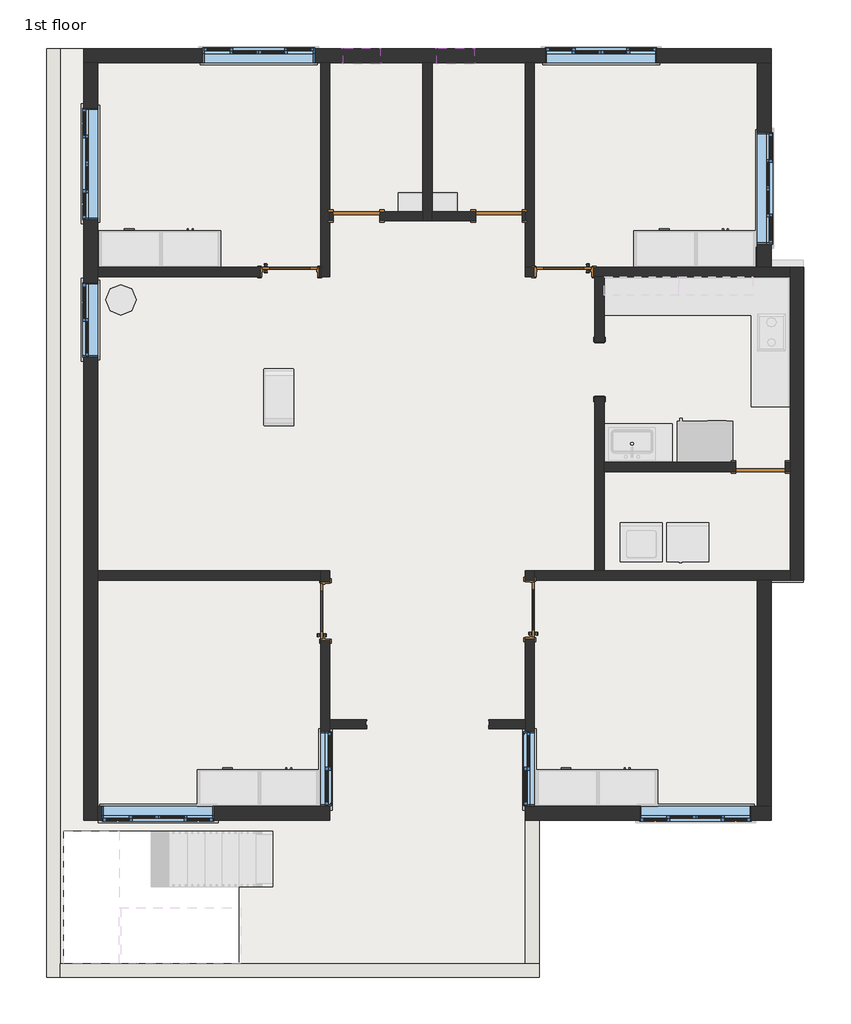
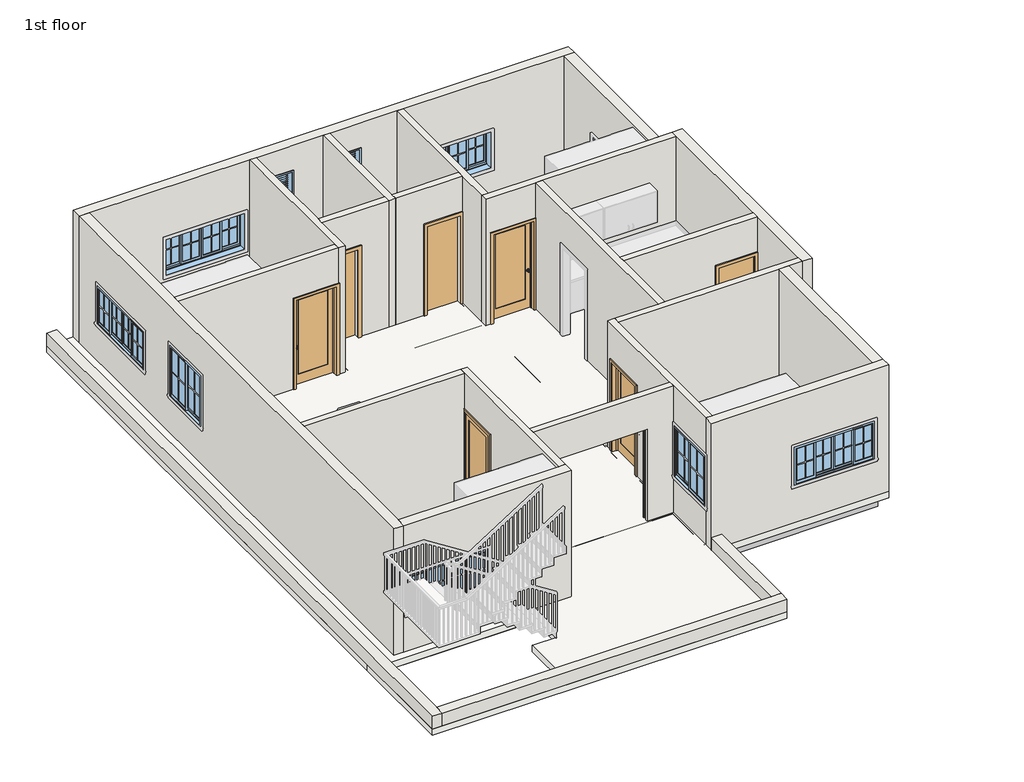
# One storey, part 1 of 4: 24 walls, 11 windows, 7 beams, 7 doors, 1 slab.
"""IFC4 building model written with IfcOpenShell, lengths in millimetres."""

from ifc_helpers import new_model, si_unit, frame, origin, place, context, project, spatial, polyline, outline, extrude, faceted_brep, transform, mapped, element, save
from components import door_010cc4d9, door_5a860750, door_e2b13fe9, door_a9addea7, door_bb092f7c, window_f2d8fef0, window_c1e3dfc0, window_49fe3060, window_58cce754

model = new_model("IFC4")

# Units and contexts
model_context = context("Model", 3, world=origin())
ifc_project = project(units=[si_unit("LENGTHUNIT", "METRE", prefix="MILLI")], contexts=[model_context])

# Site, building, storey
site = spatial("IfcSite", under=ifc_project)
building = spatial("IfcBuilding", under=site)
storey = spatial("IfcBuildingStorey", under=building, Name="1st floor", Elevation=3810.0)

# Beams
placement = place(None, origin())
element("IfcBeam", 1, ObjectType="Concrete-Rectangular Beam", at=placement, inside=storey, context=model_context, shape_type="SweptSolid", body=[
    extrude(outline(polyline([(-1593.2124084, 1316.1961804), (-1364.6124084, 1316.1961804), (-1364.6124084, -2163.6038196), (-1593.2124084, -2163.6038196), (-1593.2124084, 1316.1961804)])), frame((0.0, 0.0, 3505.2), z_axis=(0.0, 0.0, 1.0), x_axis=(1.0, 0.0, 0.0)), (0.0, 0.0, 1.0), 304.8),
])
element("IfcBeam", 2, ObjectType="Concrete-Rectangular Beam", at=placement, inside=storey, context=model_context, shape_type="Brep", body=[
    faceted_brep([(-1593.2124084, -2201.7038196, 3810.0), (-5212.7124084, -2201.7038196, 3810.0), (-5441.3124084, -2201.7038196, 3810.0), (-5441.3124084, -2239.8038196, 3810.0), (-5174.6124084, -2239.8038196, 3810.0), (-5174.6124084, -2430.3038196, 3810.0), (-1593.2124084, -2430.3038196, 3810.0), (-1593.2124084, -2201.7038196, 3505.2), (-5212.7124084, -2201.7038196, 3505.2), (-5441.3124084, -2201.7038196, 3505.2), (-1593.2124084, -2430.3038196, 3505.2), (-5174.6124084, -2430.3038196, 3505.2), (-5174.6124084, -2239.8038196, 3505.2), (-5441.3124084, -2239.8038196, 3505.2)], [[[0, 1, 2, 3, 4, 5, 6]], [[0, 7, 8, 9, 2, 1]], [[9, 8, 7, 10, 11, 12, 13]], [[10, 6, 5, 11]], [[7, 0, 6, 10]], [[2, 9, 13, 3]], [[12, 4, 3, 13]], [[4, 12, 11, 5]]]),
])
element("IfcBeam", 3, ObjectType="Concrete-Rectangular Beam", at=placement, inside=storey, context=model_context, shape_type="Brep", body=[
    faceted_brep([(-8756.0124084, -2468.4038196, 3810.0), (-8756.0124084, -2239.8038196, 3810.0), (-8794.1124084, -2239.8038196, 3810.0), (-12413.6124084, -2239.8038196, 3810.0), (-12413.6124084, -2468.4038196, 3810.0), (-8756.0124084, -2239.8038196, 3505.2), (-8794.1124084, -2239.8038196, 3505.2), (-12413.6124084, -2239.8038196, 3505.2), (-8756.0124084, -2468.4038196, 3505.2), (-12413.6124084, -2468.4038196, 3505.2)], [[[0, 1, 2, 3, 4]], [[1, 5, 6, 7, 3, 2]], [[5, 8, 9, 7, 6]], [[8, 0, 4, 9]], [[1, 0, 8, 5]], [[4, 3, 7, 9]]]),
])
element("IfcBeam", 4, ObjectType="Concrete-Rectangular Beam", at=placement, inside=storey, context=model_context, shape_type="SweptSolid", body=[
    extrude(outline(polyline([(-12642.2124084, 9875.9961804), (-12413.6124084, 9875.9961804), (-12413.6124084, 6751.7961804), (-12642.2124084, 6751.7961804), (-12642.2124084, 9875.9961804)])), frame((0.0, 0.0, 3505.2), z_axis=(0.0, 0.0, 1.0), x_axis=(1.0, 0.0, 0.0)), (0.0, 0.0, 1.0), 304.8),
    extrude(outline(polyline([(-12413.6124084, -2163.6038196), (-12642.2124084, -2163.6038196), (-12642.2124084, 1392.3961804), (-12413.6124084, 1392.3961804), (-12413.6124084, -2163.6038196)])), frame((0.0, 0.0, 3505.2), z_axis=(0.0, 0.0, 1.0), x_axis=(1.0, 0.0, 0.0)), (0.0, 0.0, 1.0), 304.8),
    extrude(outline(polyline([(-12413.6124084, 1697.1961804), (-12642.2124084, 1697.1961804), (-12642.2124084, 6446.9961804), (-12413.6124084, 6446.9961804), (-12413.6124084, 1697.1961804)])), frame((0.0, 0.0, 3505.2), z_axis=(0.0, 0.0, 1.0), x_axis=(1.0, 0.0, 0.0)), (0.0, 0.0, 1.0), 304.8),
])
element("IfcBeam", 5, ObjectType="Concrete-Rectangular Beam", at=placement, inside=storey, context=model_context, shape_type="Brep", body=[
    faceted_brep([(-843.9124084, 1659.0961804, 3810.0), (-843.9124084, 1430.4961804, 3810.0), (-843.9124084, 1430.4961804, 3505.2), (-843.9124084, 1659.0961804, 3505.2), (-5098.4124084, 1659.0961804, 3810.0), (-5098.4124084, 1468.5961804, 3810.0), (-5403.2124084, 1468.5961804, 3810.0), (-5403.2124084, 1659.0961804, 3810.0), (-5441.3124084, 1659.0961804, 3810.0), (-8565.5124084, 1659.0961804, 3810.0), (-8603.6124084, 1659.0961804, 3810.0), (-8603.6124084, 1468.5961804, 3810.0), (-8908.4124084, 1468.5961804, 3810.0), (-8908.4124084, 1659.0961804, 3810.0), (-12413.6124084, 1659.0961804, 3810.0), (-12413.6124084, 1430.4961804, 3810.0), (-8794.1124084, 1430.4961804, 3810.0), (-8565.5124084, 1430.4961804, 3810.0), (-5441.3124084, 1430.4961804, 3810.0), (-5212.7124084, 1430.4961804, 3810.0), (-1593.2124084, 1430.4961804, 3810.0), (-1593.2124084, 1620.9961804, 3810.0), (-1364.6124084, 1620.9961804, 3810.0), (-1364.6124084, 1430.4961804, 3810.0), (-1364.6124084, 1430.4961804, 3505.2), (-1364.6124084, 1620.9961804, 3505.2), (-1593.2124084, 1620.9961804, 3505.2), (-1593.2124084, 1430.4961804, 3505.2), (-5212.7124084, 1430.4961804, 3505.2), (-5441.3124084, 1430.4961804, 3505.2), (-8565.5124084, 1430.4961804, 3505.2), (-8794.1124084, 1430.4961804, 3505.2), (-12413.6124084, 1430.4961804, 3505.2), (-12413.6124084, 1659.0961804, 3505.2), (-8908.4124084, 1659.0961804, 3505.2), (-8908.4124084, 1468.5961804, 3505.2), (-8603.6124084, 1468.5961804, 3505.2), (-8603.6124084, 1659.0961804, 3505.2), (-8565.5124084, 1659.0961804, 3505.2), (-5441.3124084, 1659.0961804, 3505.2), (-5403.2124084, 1659.0961804, 3505.2), (-5403.2124084, 1468.5961804, 3505.2), (-5098.4124084, 1468.5961804, 3505.2), (-5098.4124084, 1659.0961804, 3505.2)], [[[0, 1, 2, 3]], [[1, 0, 4, 5, 6, 7, 8, 9, 10, 11, 12, 13, 14, 15, 16, 17, 18, 19, 20, 21, 22, 23]], [[2, 1, 23, 24]], [[3, 2, 24, 25, 26, 27, 28, 29, 30, 31, 32, 33, 34, 35, 36, 37, 38, 39, 40, 41, 42, 43]], [[0, 3, 43, 4]], [[15, 14, 33, 32]], [[22, 25, 24, 23]], [[26, 21, 20, 27]], [[21, 26, 25, 22]], [[15, 32, 31, 30, 29, 28, 27, 20, 19, 18, 17, 16]], [[36, 11, 10, 37]], [[11, 36, 35, 12]], [[12, 35, 34, 13]], [[33, 14, 13, 34]], [[42, 5, 4, 43]], [[5, 42, 41, 6]], [[6, 41, 40, 7]], [[37, 10, 9, 8, 7, 40, 39, 38]]]),
])
element("IfcBeam", 6, ObjectType="Concrete-Rectangular Beam", at=placement, inside=storey, context=model_context, shape_type="Brep", body=[
    faceted_brep([(-8794.1124084, -2239.8038196, 3810.0), (-8756.0124084, -2239.8038196, 3810.0), (-8565.5124084, -2239.8038196, 3810.0), (-8565.5124084, -1007.9038196, 3810.0), (-8565.5124084, -779.3038196, 3810.0), (-8565.5124084, 1430.4961804, 3810.0), (-8794.1124084, 1430.4961804, 3810.0), (-8794.1124084, -2239.8038196, 3505.2), (-8794.1124084, 1430.4961804, 3505.2), (-8565.5124084, -2239.8038196, 3505.2), (-8756.0124084, -2239.8038196, 3505.2), (-8565.5124084, 1430.4961804, 3505.2), (-8565.5124084, -779.3038196, 3505.2), (-8565.5124084, -1007.9038196, 3505.2)], [[[0, 1, 2, 3, 4, 5, 6]], [[7, 0, 6, 8]], [[9, 10, 7, 8, 11, 12, 13]], [[11, 5, 4, 3, 2, 9, 13, 12]], [[2, 1, 0, 7, 10, 9]], [[5, 11, 8, 6]]]),
    faceted_brep([(-8794.1124084, 9914.0961804, 3810.0), (-8565.5124084, 9914.0961804, 3810.0), (-8565.5124084, 9914.0961804, 3505.2), (-8794.1124084, 9914.0961804, 3505.2), (-8794.1124084, 6713.6961804, 3810.0), (-8794.1124084, 6713.6961804, 3505.2), (-8756.0124084, 6713.6961804, 3505.2), (-8756.0124084, 6713.6961804, 3810.0), (-8756.0124084, 6751.7961804, 3810.0), (-8565.5124084, 6751.7961804, 3810.0), (-8565.5124084, 7323.2961804, 3810.0), (-8565.5124084, 7551.8961804, 3810.0), (-8565.5124084, 7551.8961804, 3505.2), (-8565.5124084, 7323.2961804, 3505.2), (-8565.5124084, 6751.7961804, 3505.2), (-8756.0124084, 6751.7961804, 3505.2)], [[[0, 1, 2, 3]], [[4, 5, 6, 7]], [[1, 0, 4, 7, 8, 9, 10, 11]], [[3, 2, 12, 13, 14, 15, 6, 5]], [[0, 3, 5, 4]], [[2, 1, 11, 10, 9, 14, 13, 12]], [[15, 8, 7, 6]], [[8, 15, 14, 9]]]),
    faceted_brep([(-8794.1124084, 6485.0961804, 3505.2), (-8794.1124084, 6485.0961804, 3810.0), (-8756.0124084, 6485.0961804, 3810.0), (-8756.0124084, 6485.0961804, 3505.2), (-8565.5124084, 1659.0961804, 3505.2), (-8565.5124084, 1659.0961804, 3810.0), (-8603.6124084, 1659.0961804, 3810.0), (-8603.6124084, 1659.0961804, 3505.2), (-8565.5124084, 6446.9961804, 3505.2), (-8565.5124084, 6446.9961804, 3810.0), (-8794.1124084, 1697.1961804, 3810.0), (-8603.6124084, 1697.1961804, 3810.0), (-8756.0124084, 6446.9961804, 3810.0), (-8794.1124084, 1697.1961804, 3505.2), (-8603.6124084, 1697.1961804, 3505.2), (-8756.0124084, 6446.9961804, 3505.2)], [[[0, 1, 2, 3]], [[4, 5, 6, 7]], [[5, 4, 8, 9]], [[2, 1, 10, 11, 6, 5, 9, 12]], [[1, 0, 13, 10]], [[8, 4, 7, 14, 13, 0, 3, 15]], [[15, 12, 9, 8]], [[12, 15, 3, 2]], [[14, 11, 10, 13]], [[11, 14, 7, 6]]]),
])
element("IfcBeam", 7, ObjectType="Concrete-Rectangular Beam", at=placement, inside=storey, context=model_context, shape_type="SweptSolid", body=[
    extrude(outline(polyline([(-5441.3124084, -779.3038196), (-5441.3124084, -1007.9038196), (-8565.5124084, -1007.9038196), (-8565.5124084, -779.3038196), (-5441.3124084, -779.3038196)])), frame((0.0, 0.0, 3505.2), z_axis=(0.0, 0.0, 1.0), x_axis=(1.0, 0.0, 0.0)), (0.0, 0.0, 1.0), 304.8),
])

# Doors
door_shape = door_010cc4d9(model_context)
element("IfcDoor", 8, ObjectType="Door-Interior-Single-1_Panel-Wood : 36\" x 84\"", at=placement, inside=storey, context=model_context, shape_type="MappedRepresentation", body=[
    mapped(door_shape, transform((-9264.0124084, 6526.3711804, 3810.0), x_axis=(1.0, 0.0, 0.0), y_axis=(0.0, 1.0, 0.0), z_axis=(0.0, 0.0, 1.0))),
])
element("IfcDoor", 9, ObjectType="Door-Interior-Single-1_Panel-Wood : 36\" x 84\"", at=placement, inside=storey, context=model_context, shape_type="MappedRepresentation", body=[
    mapped(door_shape, transform((-8682.9874084, 960.5961804, 3810.0), x_axis=(0.0, 1.0, 0.0), y_axis=(-1.0, 0.0, 0.0), z_axis=(0.0, 0.0, 1.0))),
])
door_2_shape = door_5a860750(model_context)
element("IfcDoor", 10, ObjectType="Door-Interior-Single-1_Panel-Wood : 36\" x 84\"", at=placement, inside=storey, context=model_context, shape_type="MappedRepresentation", body=[
    mapped(door_2_shape, transform((-4768.2124084, 6526.3711804, 3810.0), x_axis=(-1.0, 0.0, 0.0), y_axis=(0.0, -1.0, 0.0), z_axis=(0.0, 0.0, 1.0))),
])
element("IfcDoor", 11, ObjectType="Door-Interior-Single-1_Panel-Wood : 36\" x 84\"", at=placement, inside=storey, context=model_context, shape_type="MappedRepresentation", body=[
    mapped(door_2_shape, transform((-5323.8374084, 985.9961804, 3810.0), x_axis=(0.0, 1.0, 0.0), y_axis=(-1.0, 0.0, 0.0), z_axis=(0.0, 0.0, 1.0))),
])
door_3_shape = door_e2b13fe9(model_context)
element("IfcDoor", 12, ObjectType="Single-Flush : 30\" x 84\"", at=placement, inside=storey, context=model_context, shape_type="MappedRepresentation", body=[
    mapped(door_3_shape, transform((-8171.8124084, 7437.5961804, 3810.0), x_axis=(-1.0, 0.0, 0.0), y_axis=(0.0, -1.0, 0.0), z_axis=(0.0, 0.0, 1.0))),
])
door_4_shape = door_a9addea7(model_context)
element("IfcDoor", 13, ObjectType="Single-Flush : 30\" x 84\"", at=placement, inside=storey, context=model_context, shape_type="MappedRepresentation", body=[
    mapped(door_4_shape, transform((-5835.0124084, 7437.5961804, 3810.0), x_axis=(1.0, 0.0, 0.0), y_axis=(0.0, 1.0, 0.0), z_axis=(0.0, 0.0, 1.0))),
])
door_5_shape = door_bb092f7c(model_context)
element("IfcDoor", 14, ObjectType="Single-Flush : 32\" x 84\"", at=placement, inside=storey, context=model_context, shape_type="MappedRepresentation", body=[
    mapped(door_5_shape, transform((-1542.4124084, 3322.7961804, 3810.0), x_axis=(1.0, 0.0, 0.0), y_axis=(0.0, 1.0, 0.0), z_axis=(0.0, 0.0, 1.0))),
])

# Slab
element("IfcSlab", 15, ObjectType="Generic - 6\"", at=placement, inside=storey, context=model_context, shape_type="SweptSolid", body=[
    extrude(outline(polyline([(-1364.6124084, 10180.7961804), (-1364.6124084, 6599.3961804), (-831.2124084, 6599.3961804), (-831.2124084, 1468.5961804), (-1364.6124084, 1468.5961804), (-1364.6124084, -2468.4038196), (-5174.6124084, -2468.4038196), (-5174.6124084, -5046.5038196), (-13251.8124084, -5046.5038196), (-13251.8124084, -2468.4038196), (-13251.8124084, 10180.7961804), (-1364.6124084, 10180.7961804)]), holes=[polyline([(-9543.8120641, -3536.9669819), (-9543.8120641, -2647.9669819), (-12972.8120641, -2647.9669819), (-12972.8120641, -4817.9038196), (-10102.6120641, -4817.9038196), (-10102.6120641, -3536.9669819), (-9543.8120641, -3536.9669819)])]), frame((0.0, 0.0, 3657.6), z_axis=(0.0, 0.0, 1.0), x_axis=(1.0, 0.0, 0.0)), (0.0, 0.0, 1.0), 152.4),
])

# Walls
element("IfcWall", 16, ObjectType="Generic - 6\"", at=placement, inside=storey, context=model_context, shape_type="Brep", body=[
    faceted_brep([(-8756.0124084, 9952.1961804, 3810.0), (-8756.0124084, 6599.3961804, 3810.0), (-8756.0124084, 6446.9961804, 3810.0), (-8756.0124084, 6446.9961804, 6858.0), (-8756.0124084, 6599.3961804, 6858.0), (-8756.0124084, 9952.1961804, 6858.0), (-8603.6124084, 9952.1961804, 3810.0), (-8603.6124084, 9952.1961804, 6858.0), (-8603.6124084, 7513.7961804, 6858.0), (-8603.6124084, 7361.3961804, 6858.0), (-8603.6124084, 6446.9961804, 6858.0), (-8603.6124084, 6446.9961804, 3810.0), (-8603.6124084, 7361.3961804, 3810.0), (-8603.6124084, 7513.7961804, 3810.0)], [[[0, 1, 2, 3, 4, 5]], [[6, 7, 8, 9, 10, 11, 12, 13]], [[2, 1, 0, 6, 13, 12, 11]], [[0, 5, 7, 6]], [[3, 2, 11, 10]], [[5, 4, 3, 10, 9, 8, 7]]]),
])
element("IfcWall", 17, ObjectType="Generic - 6\"", at=placement, inside=storey, context=model_context, shape_type="SweptSolid", body=[
    extrude(outline(polyline([(3810.0, -8756.0124084), (6858.0, -8756.0124084), (6858.0, -12413.6124084), (3810.0, -12413.6124084), (3810.0, -9746.6124084), (5969.0, -9746.6124084), (5969.0, -8781.4124084), (3810.0, -8781.4124084), (3810.0, -8756.0124084)])), frame((0.0, 6446.9961804, 0.0), z_axis=(0.0, 1.0, 0.0), x_axis=(0.0, 0.0, 1.0)), (0.0, 0.0, 1.0), 152.4),
])
element("IfcWall", 18, ObjectType="Generic - 6\"", at=placement, inside=storey, context=model_context, shape_type="Brep", body=[
    faceted_brep([(-7079.6124084, 9952.1961804, 3810.0), (-7079.6124084, 7513.7961804, 3810.0), (-7079.6124084, 7361.3961804, 3810.0), (-7079.6124084, 7361.3961804, 6858.0), (-7079.6124084, 7513.7961804, 6858.0), (-7079.6124084, 9952.1961804, 6858.0), (-6927.2124084, 9952.1961804, 3810.0), (-6927.2124084, 9952.1961804, 6858.0), (-6927.2124084, 7513.7961804, 6858.0), (-6927.2124084, 7361.3961804, 6858.0), (-6927.2124084, 7361.3961804, 3810.0), (-6927.2124084, 7513.7961804, 3810.0)], [[[0, 1, 2, 3, 4, 5]], [[6, 7, 8, 9, 10, 11]], [[2, 1, 0, 6, 11, 10]], [[0, 5, 7, 6]], [[3, 2, 10, 9]], [[5, 4, 3, 9, 8, 7]]]),
])
element("IfcWall", 19, ObjectType="Generic - 6\"", at=placement, inside=storey, context=model_context, shape_type="SweptSolid", body=[
    extrude(outline(polyline([(3810.0, -7079.6124084), (6858.0, -7079.6124084), (6858.0, -8603.6124084), (3810.0, -8603.6124084), (3810.0, -8552.8124084), (5943.6, -8552.8124084), (5943.6, -7790.8124084), (3810.0, -7790.8124084), (3810.0, -7079.6124084)])), frame((0.0, 7361.3961804, 0.0), z_axis=(0.0, 1.0, 0.0), x_axis=(0.0, 0.0, 1.0)), (0.0, 0.0, 1.0), 152.4),
])
element("IfcWall", 20, ObjectType="Generic - 6\"", at=placement, inside=storey, context=model_context, shape_type="SweptSolid", body=[
    extrude(outline(polyline([(6858.0, -6927.2124084), (3810.0, -6927.2124084), (3810.0, -6216.0124084), (5943.6, -6216.0124084), (5943.6, -5454.0124084), (3810.0, -5454.0124084), (3810.0, -5403.2124084), (6858.0, -5403.2124084), (6858.0, -6927.2124084)])), frame((0.0, 7361.3961804, 0.0), z_axis=(0.0, 1.0, 0.0), x_axis=(0.0, 0.0, 1.0)), (0.0, 0.0, 1.0), 152.4),
])
element("IfcWall", 21, ObjectType="Generic - 6\"", at=placement, inside=storey, context=model_context, shape_type="Brep", body=[
    faceted_brep([(-5250.8124084, 6599.3961804, 3810.0), (-5250.8124084, 9952.1961804, 3810.0), (-5250.8124084, 9952.1961804, 6858.0), (-5250.8124084, 6599.3961804, 6858.0), (-5403.2124084, 6599.3961804, 3810.0), (-5403.2124084, 6599.3961804, 6858.0), (-5403.2124084, 7361.3961804, 6858.0), (-5403.2124084, 7513.7961804, 6858.0), (-5403.2124084, 9952.1961804, 6858.0), (-5403.2124084, 9952.1961804, 3810.0), (-5403.2124084, 7513.7961804, 3810.0), (-5403.2124084, 7361.3961804, 3810.0)], [[[0, 1, 2, 3]], [[4, 5, 6, 7, 8, 9, 10, 11]], [[1, 0, 4, 11, 10, 9]], [[2, 1, 9, 8]], [[0, 3, 5, 4]], [[3, 2, 8, 7, 6, 5]]]),
])
element("IfcWall", 22, ObjectType="Generic - 6\"", at=placement, inside=storey, context=model_context, shape_type="Brep", body=[
    faceted_brep([(-5403.2124084, 6599.3961804, 3810.0), (-5403.2124084, 6599.3961804, 6858.0), (-5250.8124084, 6599.3961804, 6858.0), (-1593.2124084, 6599.3961804, 6858.0), (-1364.6124084, 6599.3961804, 6858.0), (-1059.8124084, 6599.3961804, 6858.0), (-1059.8124084, 6599.3961804, 3810.0), (-1364.6124084, 6599.3961804, 3810.0), (-1593.2124084, 6599.3961804, 3810.0), (-4285.6124084, 6599.3961804, 3810.0), (-4285.6124084, 6599.3961804, 5969.0), (-5250.8124084, 6599.3961804, 5969.0), (-5250.8124084, 6599.3961804, 3810.0), (-1059.8124084, 6446.9961804, 6858.0), (-4107.8124084, 6446.9961804, 6858.0), (-4260.2124084, 6446.9961804, 6858.0), (-5403.2124084, 6446.9961804, 6858.0), (-5403.2124084, 6446.9961804, 3810.0), (-5250.8124084, 6446.9961804, 3810.0), (-5250.8124084, 6446.9961804, 5969.0), (-4285.6124084, 6446.9961804, 5969.0), (-4285.6124084, 6446.9961804, 3810.0), (-4260.2124084, 6446.9961804, 3810.0), (-4107.8124084, 6446.9961804, 3810.0), (-1059.8124084, 6446.9961804, 3810.0)], [[[0, 1, 2, 3, 4, 5, 6, 7, 8, 9, 10, 11, 12]], [[13, 14, 15, 16, 17, 18, 19, 20, 21, 22, 23, 24]], [[17, 0, 12, 18]], [[6, 24, 23, 22, 21, 9, 8, 7]], [[1, 0, 17, 16]], [[6, 5, 13, 24]], [[11, 19, 18, 12]], [[19, 11, 10, 20]], [[20, 10, 9, 21]], [[16, 15, 14, 13, 5, 4, 3, 2, 1]]]),
])
element("IfcWall", 23, ObjectType="Generic - 6\"", at=placement, inside=storey, context=model_context, shape_type="SweptSolid", body=[
    extrude(outline(polyline([(-8756.0124084, 1468.5961804), (-12413.6124084, 1468.5961804), (-12413.6124084, 1620.9961804), (-8756.0124084, 1620.9961804), (-8756.0124084, 1468.5961804)])), frame((0.0, 0.0, 3810.0), z_axis=(0.0, 0.0, 1.0), x_axis=(1.0, 0.0, 0.0)), (0.0, 0.0, 1.0), 3048.0),
])
element("IfcWall", 24, ObjectType="Generic - 6\"", at=placement, inside=storey, context=model_context, shape_type="Brep", body=[
    faceted_brep([(-5403.2124084, -2239.8038196, 3810.0), (-5403.2124084, -2239.8038196, 6858.0), (-5403.2124084, -969.8038196, 6858.0), (-5403.2124084, -817.4038196, 6858.0), (-5403.2124084, 1620.9961804, 6858.0), (-5403.2124084, 1620.9961804, 3810.0), (-5403.2124084, 1468.5961804, 3810.0), (-5403.2124084, 1468.5961804, 5969.0), (-5403.2124084, 503.3961804, 5969.0), (-5403.2124084, 503.3961804, 3810.0), (-5403.2124084, -817.4038196, 3810.0), (-5403.2124084, -969.8038196, 3810.0), (-5403.2124084, -1014.2538196, 4724.4), (-5403.2124084, -1014.2538196, 5943.6), (-5403.2124084, -2233.4538196, 5943.6), (-5403.2124084, -2233.4538196, 4724.4), (-5250.8124084, -2239.8038196, 6858.0), (-5250.8124084, -2239.8038196, 3810.0), (-5250.8124084, 503.3961804, 3810.0), (-5250.8124084, 503.3961804, 5969.0), (-5250.8124084, 1468.5961804, 5969.0), (-5250.8124084, 1468.5961804, 3810.0), (-5250.8124084, 1620.9961804, 3810.0), (-5250.8124084, 1620.9961804, 6858.0), (-5250.8124084, 1468.5961804, 6858.0), (-5250.8124084, -1014.2538196, 5943.6), (-5250.8124084, -1014.2538196, 4724.4), (-5250.8124084, -2233.4538196, 4724.4), (-5250.8124084, -2233.4538196, 5943.6)], [[[0, 1, 2, 3, 4, 5, 6, 7, 8, 9, 10, 11], [12, 13, 14, 15]], [[16, 17, 18, 19, 20, 21, 22, 23, 24], [25, 26, 27, 28]], [[17, 0, 11, 10, 9, 18]], [[5, 22, 21, 6]], [[1, 0, 17, 16]], [[5, 4, 23, 22]], [[20, 7, 6, 21]], [[7, 20, 19, 8]], [[8, 19, 18, 9]], [[25, 13, 12, 26]], [[26, 12, 15, 27]], [[27, 15, 14, 28]], [[13, 25, 28, 14]], [[4, 3, 2, 1, 16, 24, 23]]]),
])
element("IfcWall", 25, ObjectType="Generic - 6\"", at=placement, inside=storey, context=model_context, shape_type="Brep", body=[
    faceted_brep([(-8756.0124084, 1620.9961804, 3810.0), (-8756.0124084, 1468.5961804, 3810.0), (-8756.0124084, 1443.1961804, 3810.0), (-8756.0124084, 1443.1961804, 5969.0), (-8756.0124084, 477.9961804, 5969.0), (-8756.0124084, 477.9961804, 3810.0), (-8756.0124084, -2239.8038196, 3810.0), (-8756.0124084, -2239.8038196, 6858.0), (-8756.0124084, 1468.5961804, 6858.0), (-8756.0124084, 1620.9961804, 6858.0), (-8756.0124084, -2233.4538196, 5943.6), (-8756.0124084, -2233.4538196, 4724.4), (-8756.0124084, -1014.2538196, 4724.4), (-8756.0124084, -1014.2538196, 5943.6), (-8603.6124084, 1443.1961804, 3810.0), (-8603.6124084, 1620.9961804, 3810.0), (-8603.6124084, 1620.9961804, 6858.0), (-8603.6124084, -817.4038196, 6858.0), (-8603.6124084, -969.8038196, 6858.0), (-8603.6124084, -2239.8038196, 6858.0), (-8603.6124084, -2239.8038196, 3810.0), (-8603.6124084, -969.8038196, 3810.0), (-8603.6124084, -817.4038196, 3810.0), (-8603.6124084, 477.9961804, 3810.0), (-8603.6124084, 477.9961804, 5969.0), (-8603.6124084, 1443.1961804, 5969.0), (-8603.6124084, -2233.4538196, 4724.4), (-8603.6124084, -2233.4538196, 5943.6), (-8603.6124084, -1014.2538196, 5943.6), (-8603.6124084, -1014.2538196, 4724.4)], [[[0, 1, 2, 3, 4, 5, 6, 7, 8, 9], [10, 11, 12, 13]], [[14, 15, 16, 17, 18, 19, 20, 21, 22, 23, 24, 25], [26, 27, 28, 29]], [[6, 5, 23, 22, 21, 20]], [[2, 1, 0, 15, 14]], [[25, 3, 2, 14]], [[3, 25, 24, 4]], [[4, 24, 23, 5]], [[0, 9, 16, 15]], [[10, 27, 26, 11]], [[11, 26, 29, 12]], [[12, 29, 28, 13]], [[27, 10, 13, 28]], [[9, 8, 7, 19, 18, 17, 16]], [[7, 6, 20, 19]]]),
])
element("IfcWall", 26, ObjectType="Generic - 6\"", at=placement, inside=storey, context=model_context, shape_type="Brep", body=[
    faceted_brep([(-4260.2124084, 6446.9961804, 6858.0), (-4260.2124084, 6446.9961804, 3810.0), (-4260.2124084, 5380.1961804, 3810.0), (-4260.2124084, 5380.1961804, 5943.6), (-4260.2124084, 4465.7961804, 5943.6), (-4260.2124084, 4465.7961804, 3810.0), (-4260.2124084, 1620.9961804, 3810.0), (-4260.2124084, 1620.9961804, 6858.0), (-4107.8124084, 6446.9961804, 3810.0), (-4107.8124084, 6446.9961804, 6858.0), (-4107.8124084, 3398.9961804, 6858.0), (-4107.8124084, 3246.5961804, 6858.0), (-4107.8124084, 1620.9961804, 6858.0), (-4107.8124084, 1620.9961804, 3810.0), (-4107.8124084, 3246.5961804, 3810.0), (-4107.8124084, 3398.9961804, 3810.0), (-4107.8124084, 4465.7961804, 3810.0), (-4107.8124084, 4465.7961804, 5943.6), (-4107.8124084, 5380.1961804, 5943.6), (-4107.8124084, 5380.1961804, 3810.0)], [[[0, 1, 2, 3, 4, 5, 6, 7]], [[8, 9, 10, 11, 12, 13, 14, 15, 16, 17, 18, 19]], [[1, 8, 19, 2]], [[13, 6, 5, 16, 15, 14]], [[1, 0, 9, 8]], [[7, 6, 13, 12]], [[4, 17, 16, 5]], [[18, 3, 2, 19]], [[17, 4, 3, 18]], [[0, 7, 12, 11, 10, 9]]]),
])
element("IfcWall", 27, ObjectType="Generic - 6\"", at=placement, inside=storey, context=model_context, shape_type="SweptSolid", body=[
    extrude(outline(polyline([(6858.0, -4107.8124084), (3810.0, -4107.8124084), (3810.0, -1948.8124084), (5943.6, -1948.8124084), (5943.6, -1136.0124084), (3810.0, -1136.0124084), (3810.0, -1059.8124084), (6858.0, -1059.8124084), (6858.0, -4107.8124084)])), frame((0.0, 3246.5961804, 0.0), z_axis=(0.0, 1.0, 0.0), x_axis=(0.0, 0.0, 1.0)), (0.0, 0.0, 1.0), 152.4),
])
element("IfcWall", 28, ObjectType="Generic - 6\"", at=placement, inside=storey, context=model_context, shape_type="Brep", body=[
    faceted_brep([(-5250.8124084, 1468.5961804, 3810.0), (-1593.2124084, 1468.5961804, 3810.0), (-1364.6124084, 1468.5961804, 3810.0), (-1059.8124084, 1468.5961804, 3810.0), (-1059.8124084, 1468.5961804, 6858.0), (-1364.6124084, 1468.5961804, 6858.0), (-1593.2124084, 1468.5961804, 6858.0), (-5250.8124084, 1468.5961804, 6858.0), (-5250.8124084, 1620.9961804, 3810.0), (-5250.8124084, 1620.9961804, 6858.0), (-4260.2124084, 1620.9961804, 6858.0), (-4107.8124084, 1620.9961804, 6858.0), (-1059.8124084, 1620.9961804, 6858.0), (-1059.8124084, 1620.9961804, 3810.0), (-4107.8124084, 1620.9961804, 3810.0), (-4260.2124084, 1620.9961804, 3810.0)], [[[0, 1, 2, 3, 4, 5, 6, 7]], [[8, 9, 10, 11, 12, 13, 14, 15]], [[3, 2, 1, 0, 8, 15, 14, 13]], [[4, 3, 13, 12]], [[0, 7, 9, 8]], [[7, 6, 5, 4, 12, 11, 10, 9]]]),
])
element("IfcWall", 29, ObjectType="Generic - 6\"", at=placement, inside=storey, context=model_context, shape_type="Brep", body=[
    faceted_brep([(-5403.2124084, -969.8038196, 3810.0), (-5403.2124084, -969.8038196, 6858.0), (-8603.6124084, -969.8038196, 6858.0), (-8603.6124084, -969.8038196, 3810.0), (-8003.4124084, -969.8038196, 3810.0), (-8003.4124084, -969.8038196, 6019.0), (-6003.4124084, -969.8038196, 6019.0), (-6003.4124084, -969.8038196, 3810.0), (-5403.2124084, -817.4038196, 6858.0), (-5403.2124084, -817.4038196, 3810.0), (-6003.4124084, -817.4038196, 3810.0), (-6003.4124084, -817.4038196, 6019.0), (-8003.4124084, -817.4038196, 6019.0), (-8003.4124084, -817.4038196, 3810.0), (-8603.6124084, -817.4038196, 3810.0), (-8603.6124084, -817.4038196, 6858.0), (-8003.4124084, -837.4038196, 3810.0), (-8018.4124084, -837.4038196, 3810.0), (-8018.4124084, -907.4038196, 3810.0), (-8003.4124084, -907.4038196, 3810.0), (-6003.4124084, -907.4038196, 3810.0), (-5988.4124084, -907.4038196, 3810.0), (-5988.4124084, -837.4038196, 3810.0), (-6003.4124084, -837.4038196, 3810.0), (-6003.4124084, -837.4038196, 6019.0), (-8003.4124084, -837.4038196, 6019.0), (-8003.4124084, -907.4038196, 6019.0), (-6003.4124084, -907.4038196, 6019.0), (-8018.4124084, -907.4038196, 6034.0), (-5988.4124084, -907.4038196, 6034.0), (-5988.4124084, -837.4038196, 6034.0), (-8018.4124084, -837.4038196, 6034.0)], [[[0, 1, 2, 3, 4, 5, 6, 7]], [[8, 9, 10, 11, 12, 13, 14, 15]], [[3, 14, 13, 16, 17, 18, 19, 4]], [[9, 0, 7, 20, 21, 22, 23, 10]], [[1, 0, 9, 8]], [[3, 2, 15, 14]], [[24, 25, 12, 11]], [[26, 27, 6, 5]], [[19, 26, 5, 4]], [[27, 20, 7, 6]], [[27, 26, 19, 18, 28, 29, 21, 20]], [[21, 29, 30, 22]], [[25, 24, 23, 22, 30, 31, 17, 16]], [[23, 24, 11, 10]], [[25, 16, 13, 12]], [[28, 18, 17, 31]], [[29, 28, 31, 30]], [[2, 1, 8, 15]]]),
])
element("IfcWall", 30, ObjectType="Generic - 9\"", at=placement, inside=storey, context=model_context, shape_type="Brep", body=[
    faceted_brep([(-12642.2124084, 9952.1961804, 3810.0), (-12413.6124084, 9952.1961804, 3810.0), (-8756.0124084, 9952.1961804, 3810.0), (-8603.6124084, 9952.1961804, 3810.0), (-7079.6124084, 9952.1961804, 3810.0), (-6927.2124084, 9952.1961804, 3810.0), (-5403.2124084, 9952.1961804, 3810.0), (-5250.8124084, 9952.1961804, 3810.0), (-1593.2124084, 9952.1961804, 3810.0), (-1364.6124084, 9952.1961804, 3810.0), (-1364.6124084, 9952.1961804, 6858.0), (-1593.2124084, 9952.1961804, 6858.0), (-5250.8124084, 9952.1961804, 6858.0), (-5403.2124084, 9952.1961804, 6858.0), (-6927.2124084, 9952.1961804, 6858.0), (-7079.6124084, 9952.1961804, 6858.0), (-8603.6124084, 9952.1961804, 6858.0), (-8756.0124084, 9952.1961804, 6858.0), (-12413.6124084, 9952.1961804, 6858.0), (-12642.2124084, 9952.1961804, 6858.0), (-3244.2124084, 9952.1961804, 5638.8), (-3244.2124084, 9952.1961804, 4724.4), (-5073.0124084, 9952.1961804, 4724.4), (-5073.0124084, 9952.1961804, 5638.8), (-8857.6124084, 9952.1961804, 5638.8), (-8857.6124084, 9952.1961804, 4724.4), (-10686.4124084, 9952.1961804, 4724.4), (-10686.4124084, 9952.1961804, 5638.8), (-8387.7124084, 9952.1961804, 5638.8), (-8387.7124084, 9952.1961804, 6248.4), (-7778.1124084, 9952.1961804, 6248.4), (-7778.1124084, 9952.1961804, 5638.8), (-6851.0124084, 9952.1961804, 5638.8), (-6851.0124084, 9952.1961804, 6248.4), (-6241.4124084, 9952.1961804, 6248.4), (-6241.4124084, 9952.1961804, 5638.8), (-1364.6124084, 10180.7961804, 3810.0), (-12642.2124084, 10180.7961804, 3810.0), (-12642.2124084, 10180.7961804, 6858.0), (-1364.6124084, 10180.7961804, 6858.0), (-3244.2124084, 10180.7961804, 4724.4), (-3244.2124084, 10180.7961804, 5638.8), (-5073.0124084, 10180.7961804, 5638.8), (-5073.0124084, 10180.7961804, 4724.4), (-8857.6124084, 10180.7961804, 4724.4), (-8857.6124084, 10180.7961804, 5638.8), (-10686.4124084, 10180.7961804, 5638.8), (-10686.4124084, 10180.7961804, 4724.4), (-8387.7124084, 10180.7961804, 6248.4), (-8387.7124084, 10180.7961804, 5638.8), (-7778.1124084, 10180.7961804, 5638.8), (-7778.1124084, 10180.7961804, 6248.4), (-6851.0124084, 10180.7961804, 6248.4), (-6851.0124084, 10180.7961804, 5638.8), (-6241.4124084, 10180.7961804, 5638.8), (-6241.4124084, 10180.7961804, 6248.4)], [[[0, 1, 2, 3, 4, 5, 6, 7, 8, 9, 10, 11, 12, 13, 14, 15, 16, 17, 18, 19], [20, 21, 22, 23], [24, 25, 26, 27], [28, 29, 30, 31], [32, 33, 34, 35]], [[36, 37, 38, 39], [40, 41, 42, 43], [44, 45, 46, 47], [48, 49, 50, 51], [52, 53, 54, 55]], [[9, 8, 7, 6, 5, 4, 3, 2, 1, 0, 37, 36]], [[0, 19, 38, 37]], [[10, 9, 36, 39]], [[20, 41, 40, 21]], [[21, 40, 43, 22]], [[22, 43, 42, 23]], [[41, 20, 23, 42]], [[24, 45, 44, 25]], [[25, 44, 47, 26]], [[46, 27, 26, 47]], [[45, 24, 27, 46]], [[49, 48, 29, 28]], [[50, 49, 28, 31]], [[51, 50, 31, 30]], [[48, 51, 30, 29]], [[53, 52, 33, 32]], [[54, 53, 32, 35]], [[55, 54, 35, 34]], [[52, 55, 34, 33]], [[19, 18, 17, 16, 15, 14, 13, 12, 11, 10, 39, 38]]]),
])
element("IfcWall", 31, ObjectType="Generic - 9\"", at=placement, inside=storey, context=model_context, shape_type="Brep", body=[
    faceted_brep([(-12642.2124084, 9952.1961804, 3810.0), (-12642.2124084, -2468.4038196, 3810.0), (-12642.2124084, -2468.4038196, 6858.0), (-12642.2124084, 9952.1961804, 6858.0), (-12642.2124084, 5126.1961804, 5943.6), (-12642.2124084, 5126.1961804, 4724.4), (-12642.2124084, 6345.3961804, 4724.4), (-12642.2124084, 6345.3961804, 5943.6), (-12642.2124084, 9209.2461804, 4724.4), (-12642.2124084, 9209.2461804, 5638.8), (-12642.2124084, 7380.4461804, 5638.8), (-12642.2124084, 7380.4461804, 4724.4), (-12413.6124084, -2468.4038196, 3810.0), (-12413.6124084, -2239.8038196, 3810.0), (-12413.6124084, 1468.5961804, 3810.0), (-12413.6124084, 1620.9961804, 3810.0), (-12413.6124084, 6446.9961804, 3810.0), (-12413.6124084, 6599.3961804, 3810.0), (-12413.6124084, 9952.1961804, 3810.0), (-12413.6124084, 9952.1961804, 6858.0), (-12413.6124084, 6599.3961804, 6858.0), (-12413.6124084, 6446.9961804, 6858.0), (-12413.6124084, 1620.9961804, 6858.0), (-12413.6124084, 1468.5961804, 6858.0), (-12413.6124084, -2239.8038196, 6858.0), (-12413.6124084, -2468.4038196, 6858.0), (-12413.6124084, 5126.1961804, 4724.4), (-12413.6124084, 5126.1961804, 5943.6), (-12413.6124084, 6345.3961804, 5943.6), (-12413.6124084, 6345.3961804, 4724.4), (-12413.6124084, 9209.2461804, 5638.8), (-12413.6124084, 9209.2461804, 4724.4), (-12413.6124084, 7380.4461804, 4724.4), (-12413.6124084, 7380.4461804, 5638.8)], [[[0, 1, 2, 3], [4, 5, 6, 7], [8, 9, 10, 11]], [[12, 13, 14, 15, 16, 17, 18, 19, 20, 21, 22, 23, 24, 25], [26, 27, 28, 29], [30, 31, 32, 33]], [[1, 0, 18, 17, 16, 15, 14, 13, 12]], [[0, 3, 19, 18]], [[2, 1, 12, 25]], [[4, 27, 26, 5]], [[5, 26, 29, 6]], [[6, 29, 28, 7]], [[30, 9, 8, 31]], [[31, 8, 11, 32]], [[10, 33, 32, 11]], [[9, 30, 33, 10]], [[27, 4, 7, 28]], [[3, 2, 25, 24, 23, 22, 21, 20, 19]]]),
])
element("IfcWall", 32, ObjectType="Generic - 9\"", at=placement, inside=storey, context=model_context, shape_type="SweptSolid", body=[
    extrude(outline(polyline([(9952.1961804, 3810.0), (6599.3961804, 3810.0), (6599.3961804, 6858.0), (9952.1961804, 6858.0), (9952.1961804, 3810.0)]), holes=[polyline([(6980.3961804, 5638.8), (6980.3961804, 4724.4), (8809.1961804, 4724.4), (8809.1961804, 5638.8), (6980.3961804, 5638.8)])]), frame((-1593.2124084, 0.0, 0.0), z_axis=(1.0, 0.0, 0.0), x_axis=(0.0, 1.0, 0.0)), (0.0, 0.0, 1.0), 228.6),
])
element("IfcWall", 33, ObjectType="Generic - 9\"", at=placement, inside=storey, context=model_context, shape_type="Brep", body=[
    faceted_brep([(-12413.6124084, -2468.4038196, 3810.0), (-8603.6124084, -2468.4038196, 3810.0), (-8603.6124084, -2468.4038196, 6858.0), (-12413.6124084, -2468.4038196, 6858.0), (-12337.4124084, -2468.4038196, 4724.4), (-12337.4124084, -2468.4038196, 5638.8), (-10508.6124084, -2468.4038196, 5638.8), (-10508.6124084, -2468.4038196, 4724.4), (-8603.6124084, -2239.8038196, 3810.0), (-8756.0124084, -2239.8038196, 3810.0), (-12413.6124084, -2239.8038196, 3810.0), (-12413.6124084, -2239.8038196, 6858.0), (-8756.0124084, -2239.8038196, 6858.0), (-8603.6124084, -2239.8038196, 6858.0), (-12337.4124084, -2239.8038196, 5638.8), (-12337.4124084, -2239.8038196, 4724.4), (-10508.6124084, -2239.8038196, 4724.4), (-10508.6124084, -2239.8038196, 5638.8)], [[[0, 1, 2, 3], [4, 5, 6, 7]], [[8, 9, 10, 11, 12, 13], [14, 15, 16, 17]], [[1, 0, 10, 9, 8]], [[0, 3, 11, 10]], [[14, 5, 4, 15]], [[15, 4, 7, 16]], [[16, 7, 6, 17]], [[5, 14, 17, 6]], [[3, 2, 13, 12, 11]], [[2, 1, 8, 13]]]),
])
element("IfcWall", 34, ObjectType="Generic - 9\"", at=placement, inside=storey, context=model_context, shape_type="SweptSolid", body=[
    extrude(outline(polyline([(-1593.2124084, -2239.8038196), (-1593.2124084, 1468.5961804), (-1364.6124084, 1468.5961804), (-1364.6124084, -2239.8038196), (-1593.2124084, -2239.8038196)])), frame((0.0, 0.0, 3810.0), z_axis=(0.0, 0.0, 1.0), x_axis=(1.0, 0.0, 0.0)), (0.0, 0.0, 1.0), 3048.0),
])
element("IfcWall", 35, ObjectType="Generic - 9\"", at=placement, inside=storey, context=model_context, shape_type="Brep", body=[
    faceted_brep([(-1059.8124084, 6599.3961804, 3810.0), (-1059.8124084, 6446.9961804, 3810.0), (-1059.8124084, 3398.9961804, 3810.0), (-1059.8124084, 3246.5961804, 3810.0), (-1059.8124084, 1620.9961804, 3810.0), (-1059.8124084, 1468.5961804, 3810.0), (-1059.8124084, 1468.5961804, 6858.0), (-1059.8124084, 1620.9961804, 6858.0), (-1059.8124084, 3246.5961804, 6858.0), (-1059.8124084, 3398.9961804, 6858.0), (-1059.8124084, 6446.9961804, 6858.0), (-1059.8124084, 6599.3961804, 6858.0), (-831.2124084, 6599.3961804, 3810.0), (-831.2124084, 6599.3961804, 6858.0), (-831.2124084, 1468.5961804, 6858.0), (-831.2124084, 1468.5961804, 3810.0)], [[[0, 1, 2, 3, 4, 5, 6, 7, 8, 9, 10, 11]], [[12, 13, 14, 15]], [[5, 4, 3, 2, 1, 0, 12, 15]], [[0, 11, 13, 12]], [[6, 5, 15, 14]], [[11, 10, 9, 8, 7, 6, 14, 13]]]),
])
element("IfcWall", 36, ObjectType="Generic - 9\"", at=placement, inside=storey, context=model_context, shape_type="Brep", body=[
    faceted_brep([(-5403.2124084, -2468.4038196, 3810.0), (-5174.6124084, -2468.4038196, 3810.0), (-1364.6124084, -2468.4038196, 3810.0), (-1364.6124084, -2468.4038196, 6858.0), (-5174.6124084, -2468.4038196, 6858.0), (-5403.2124084, -2468.4038196, 6858.0), (-5403.2124084, -2468.4038196, 4114.8), (-3523.6124084, -2468.4038196, 4724.4), (-3523.6124084, -2468.4038196, 5638.8), (-1694.8124084, -2468.4038196, 5638.8), (-1694.8124084, -2468.4038196, 4724.4), (-1364.6124084, -2239.8038196, 3810.0), (-1593.2124084, -2239.8038196, 3810.0), (-5250.8124084, -2239.8038196, 3810.0), (-5403.2124084, -2239.8038196, 3810.0), (-5403.2124084, -2239.8038196, 6858.0), (-5250.8124084, -2239.8038196, 6858.0), (-1593.2124084, -2239.8038196, 6858.0), (-1364.6124084, -2239.8038196, 6858.0), (-3523.6124084, -2239.8038196, 5638.8), (-3523.6124084, -2239.8038196, 4724.4), (-1694.8124084, -2239.8038196, 4724.4), (-1694.8124084, -2239.8038196, 5638.8)], [[[0, 1, 2, 3, 4, 5, 6], [7, 8, 9, 10]], [[11, 12, 13, 14, 15, 16, 17, 18], [19, 20, 21, 22]], [[2, 1, 0, 14, 13, 12, 11]], [[3, 2, 11, 18]], [[19, 8, 7, 20]], [[20, 7, 10, 21]], [[21, 10, 9, 22]], [[8, 19, 22, 9]], [[18, 17, 16, 15, 5, 4, 3]], [[0, 6, 5, 15, 14]]]),
])
element("IfcWall", 37, ObjectType="Generic - 9\"", at=placement, inside=storey, context=model_context, shape_type="Brep", body=[
    faceted_brep([(-13251.8124084, 10180.7961804, 3810.0), (-13251.8124084, -5046.5038196, 3810.0), (-13251.8124084, -5046.5038196, 4114.8), (-13251.8124084, 10180.7961804, 4114.8), (-13023.2124084, 10180.7961804, 3810.0), (-13023.2124084, 10180.7961804, 4114.8), (-13023.2124084, -4817.9038196, 4114.8), (-13023.2124084, -5046.5038196, 4114.8), (-13023.2124084, -5046.5038196, 3810.0), (-13023.2124084, -4817.9038196, 3810.0)], [[[0, 1, 2, 3]], [[4, 5, 6, 7, 8, 9]], [[1, 0, 4, 9, 8]], [[3, 2, 7, 6, 5]], [[0, 3, 5, 4]], [[2, 1, 8, 7]]]),
])
element("IfcWall", 38, ObjectType="Generic - 9\"", at=placement, inside=storey, context=model_context, shape_type="Brep", body=[
    faceted_brep([(-13023.2124084, -5046.5038196, 3810.0), (-5174.6124084, -5046.5038196, 3810.0), (-5174.6124084, -5046.5038196, 4114.8), (-13023.2124084, -5046.5038196, 4114.8), (-13023.2124084, -4817.9038196, 3810.0), (-13023.2124084, -4817.9038196, 4114.8), (-5403.2124084, -4817.9038196, 4114.8), (-5174.6124084, -4817.9038196, 4114.8), (-5174.6124084, -4817.9038196, 3810.0), (-5403.2124084, -4817.9038196, 3810.0)], [[[0, 1, 2, 3]], [[4, 5, 6, 7, 8, 9]], [[1, 0, 4, 9, 8]], [[3, 2, 7, 6, 5]], [[0, 3, 5, 4]], [[2, 1, 8, 7]]]),
])
element("IfcWall", 39, ObjectType="Generic - 9\"", at=placement, inside=storey, context=model_context, shape_type="SweptSolid", body=[
    extrude(outline(polyline([(-5174.6124084, -2468.4038196), (-5174.6124084, -4817.9038196), (-5403.2124084, -4817.9038196), (-5403.2124084, -2468.4038196), (-5174.6124084, -2468.4038196)])), frame((0.0, 0.0, 3810.0), z_axis=(0.0, 0.0, 1.0), x_axis=(1.0, 0.0, 0.0)), (0.0, 0.0, 1.0), 304.8),
])

# Windows
window_shape = window_f2d8fef0(model_context)
element("IfcWindow", 40, ObjectType="Window-Louvers : 24\" x 24\"", at=placement, inside=storey, context=model_context, shape_type="MappedRepresentation", body=[
    mapped(window_shape, transform((-8082.9124084, 10072.8461804, 4724.4), x_axis=(1.0, 0.0, 0.0), y_axis=(0.0, 1.0, 0.0), z_axis=(0.0, 0.0, 1.0))),
])
element("IfcWindow", 41, ObjectType="Window-Louvers : 24\" x 24\"", at=placement, inside=storey, context=model_context, shape_type="MappedRepresentation", body=[
    mapped(window_shape, transform((-6546.2124084, 10072.8461804, 4724.4), x_axis=(1.0, 0.0, 0.0), y_axis=(0.0, 1.0, 0.0), z_axis=(0.0, 0.0, 1.0))),
])
window_2_shape = window_c1e3dfc0(model_context)
element("IfcWindow", 42, ObjectType="Window-Sliding-Double : 48\" x 48\"", at=placement, inside=storey, context=model_context, shape_type="MappedRepresentation", body=[
    mapped(window_2_shape, transform((-12531.7224084, 5735.7961804, 3810.0), x_axis=(0.0, -1.0, 0.0), y_axis=(1.0, 0.0, 0.0), z_axis=(0.0, 0.0, 1.0))),
])
window_3_shape = window_49fe3060(model_context)
element("IfcWindow", 43, ObjectType="Window-Sliding-Double : 48\" x 48\"", at=placement, inside=storey, context=model_context, shape_type="MappedRepresentation", body=[
    mapped(window_3_shape, transform((-8676.0024084, -1623.8538196, 3810.0), x_axis=(0.0, -1.0, 0.0), y_axis=(1.0, 0.0, 0.0), z_axis=(0.0, 0.0, 1.0))),
])
element("IfcWindow", 44, ObjectType="Window-Sliding-Double : 48\" x 48\"", at=placement, inside=storey, context=model_context, shape_type="MappedRepresentation", body=[
    mapped(window_3_shape, transform((-5330.8224084, -1623.8538196, 3810.0), x_axis=(0.0, 1.0, 0.0), y_axis=(-1.0, 0.0, 0.0), z_axis=(0.0, 0.0, 1.0))),
])
window_4_shape = window_58cce754(model_context)
element("IfcWindow", 45, ObjectType="Window-Sliding-Four : 72\" x 36\"", at=placement, inside=storey, context=model_context, shape_type="MappedRepresentation", body=[
    mapped(window_4_shape, transform((-9772.0124084, 10070.3061804, 3810.0), x_axis=(1.0, 0.0, 0.0), y_axis=(0.0, 1.0, 0.0), z_axis=(0.0, 0.0, 1.0))),
])
element("IfcWindow", 46, ObjectType="Window-Sliding-Four : 72\" x 36\"", at=placement, inside=storey, context=model_context, shape_type="MappedRepresentation", body=[
    mapped(window_4_shape, transform((-12531.7224084, 8294.8461804, 3810.0), x_axis=(0.0, 1.0, 0.0), y_axis=(-1.0, 0.0, 0.0), z_axis=(0.0, 0.0, 1.0))),
])
element("IfcWindow", 47, ObjectType="Window-Sliding-Four : 72\" x 36\"", at=placement, inside=storey, context=model_context, shape_type="MappedRepresentation", body=[
    mapped(window_4_shape, transform((-1475.1024084, 7894.7961804, 3810.0), x_axis=(0.0, -1.0, 0.0), y_axis=(1.0, 0.0, 0.0), z_axis=(0.0, 0.0, 1.0))),
])
element("IfcWindow", 48, ObjectType="Window-Sliding-Four : 72\" x 36\"", at=placement, inside=storey, context=model_context, shape_type="MappedRepresentation", body=[
    mapped(window_4_shape, transform((-4158.6124084, 10070.3061804, 3810.0), x_axis=(1.0, 0.0, 0.0), y_axis=(0.0, 1.0, 0.0), z_axis=(0.0, 0.0, 1.0))),
])
element("IfcWindow", 49, ObjectType="Window-Sliding-Four : 72\" x 36\"", at=placement, inside=storey, context=model_context, shape_type="MappedRepresentation", body=[
    mapped(window_4_shape, transform((-2609.2124084, -2357.9138196, 3810.0), x_axis=(-1.0, 0.0, 0.0), y_axis=(0.0, -1.0, 0.0), z_axis=(0.0, 0.0, 1.0))),
])
element("IfcWindow", 50, ObjectType="Window-Sliding-Four : 72\" x 36\"", at=placement, inside=storey, context=model_context, shape_type="MappedRepresentation", body=[
    mapped(window_4_shape, transform((-11423.0124084, -2357.9138196, 3810.0), x_axis=(-1.0, 0.0, 0.0), y_axis=(0.0, -1.0, 0.0), z_axis=(0.0, 0.0, 1.0))),
])

save(model, "model.ifc")

# Revit data of these elements
# Type "Concrete-Rectangular Beam"
#   Assembly Code = "B10"
#   Length [instance default] = 5' - 0"
#   b = 0' - 9"
#   h = 1' - 0"
#   Structural Material [instance default] = Concrete, Cast-in-Place gray
# Type "Door-Interior-Single-1_Panel-Wood : 36\" x 84\""
#   Type Mark = "8"
#   Assembly Code = "C1020300"
#   Analytic Construction = "Wooden"
#   Top Rail = 0' - 4 11/16"
#   Thickness = 0' - 1 3/8"
#   Thermal Resistance (R) = 2.5876 (h·ft²·°F)/BTU
#   Swing Angle [instance default] = 90.00°
#   Stiles = 0' - 4 3/4"
#   Rough Width = 3' - 2"
#   Rough Height = 7' - 1"
#   Height = 7' - 0"
#   Width = 3' - 0"
#   Heat Transfer Coefficient (U) = 0.3865 BTU/(h·ft²·°F)
#   Bottom Rail = 0' - 9 1/8"
#   Trim Material = Cherry
#   Panel Material = Cherry
#   Frame Material = Cherry
#   Door Handle Material = Aluminum
#   Visual Light Transmittance = 0
#   Solar Heat Gain Coefficient = 0
#   Wall Closure = (empty or 0)
#   Function = (empty or 0)
# Type "Single-Flush : 30\" x 84\""
#   Type Mark = "4"
#   Construction Type Id = "MDOOR"
#   Assembly Code = "C1020"
#   Analytic Construction = "Metal"
#   Thickness = 0' - 2"
#   Heat Transfer Coefficient (U) = 0.651978 BTU/(h·ft²·°F)
#   Height = 7' - 0"
#   Trim Projection Ext = 0' - 1"
#   Trim Projection Int = 0' - 1"
#   Trim Width = 0' - 3"
#   Width = 2' - 6"
#   Define Thermal Properties by = 1
#   Define Thermal Properties by = 1
#   Door Material = Door - Panel
#   Frame Material = Door - Frame
#   Visual Light Transmittance = 0
#   Solar Heat Gain Coefficient = 0
#   Function = (empty or 0)
#   Wall Closure = (empty or 0)
# Type "Single-Flush : 32\" x 84\""
#   Type Mark = "3"
#   Construction Type Id = "MDOOR"
#   Assembly Code = "C1020"
#   Analytic Construction = "Metal"
#   Thickness = 0' - 2"
#   Heat Transfer Coefficient (U) = 0.651978 BTU/(h·ft²·°F)
#   Height = 7' - 0"
#   Trim Projection Ext = 0' - 1"
#   Trim Projection Int = 0' - 1"
#   Trim Width = 0' - 3"
#   Width = 2' - 8"
#   Define Thermal Properties by = 1
#   Define Thermal Properties by = 1
#   Door Material = Door - Panel
#   Frame Material = Door - Frame
#   Visual Light Transmittance = 0
#   Solar Heat Gain Coefficient = 0
#   Function = (empty or 0)
#   Wall Closure = (empty or 0)
# Type "Generic - 6\""
#   Assembly Code = "B1010"
#   Function = 0
#   Layers, outside or top first: 0' - 6" no material (function 1)
# Type "Generic - 6\""
#   Assembly Code = "B2010"
#   Layers, outside or top first: 0' - 6" no material (function 1)
# Type "Generic - 9\""
#   Assembly Code = "B2010"
#   Layers, outside or top first: 0' - 9" no material (function 1)
# Type "Window-Louvers : 24\" x 24\""
#   Type Mark = "24"
#   Construction Type Id = "GSP4R"
#   Assembly Code = "B20"
#   Analytic Construction = "1/8 in Pilkington single glazing"
#   Visual Light Transmittance = 0.9
#   Thermal Resistance (R) = 1.53941 (h·ft²·°F)/BTU
#   Solar Heat Gain Coefficient = 0.78
#   Max Height = 1' - 11.74264"
#   Height = 2' - 0"
#   Heat Transfer Coefficient (U) = 0.6496 BTU/(h·ft²·°F)
#   Blade Width [instance default] = 1' - 10 1/2"
#   Blade Vertical Thickness = 0' - 0.35355"
#   Blade Thickness = 0' - 0 1/4"
#   Blade Spacing = 0' - 1 1/2"
#   Blade Height = 0' - 1.85355"
#   Blade Depth = 0' - 3"
#   Blade Angle = 45.00°
#   Default Sill Height = 3' - 0"
#   Trim Projection_Exterior = 0' - 0 1/2"
#   Trim Projection_Interior = 0' - 0 1/2"
#   Trim Width_Exterior = 0' - 1 1/2"
#   Trim Width_Interior = 0' - 1 1/2"
#   Width = 2' - 0"
#   Max Blade Count = 12
#   Define Thermal Properties by = 1
#   Blade Count = 12
#   Frame Material = Birch
#   Louver Material = Birch
#   Trim Exterior Material = Birch
#   Trim Interior Material = Birch
#   Wall Closure = (empty or 0)
# Type "Window-Sliding-Double : 48\" x 48\""
#   Type Mark = "23"
#   Fire Rating = "0.5h"
#   Assembly Code = "B2020100"
#   Analytic Construction = "Double glazing - domestic"
#   Window Inset [instance default] = 0' - 0"
#   Wall Thickness [instance default] = 0' - 6"
#   Visual Light Transmittance = 0.81
#   Thermal Resistance (R) = 1.8146 (h·ft²·°F)/BTU
#   Solar Heat Gain Coefficient = 0.76
#   Muntin Width = 1' - 8 5/8"
#   Muntin Height = 3' - 6 1/4"
#   Interior Wall Closure [instance default] = 0' - 2 3/4"
#   Heat Transfer Coefficient (U) = 0.5511 BTU/(h·ft²·°F)
#   Frame Extension [instance default] = 0' - 0 1/4"
#   Exterior Wall Closure [instance default] = 0' - 1 1/4"
#   Rough Width = 4' - 0 1/2"
#   Rough Height = 4' - 0 1/2"
#   Height = 4' - 0"
#   Extension Jamb [instance default] = 0' - 2 3/4"
#   Default Sill Height = 3' - 0"
#   Width = 4' - 0"
#   Interior Trim Visibility [instance default] = yes
#   Indicator Visibility [instance default] = yes
#   Exterior Trim Visibility [instance default] = yes
#   Muntin Visibility = yes
#   Extension Jamb Visibility [instance default] = yes
#   Muntin Pattern = Muntin Pattern_2x2 : Muntin Pattern_2x2
#   Interior Trim Material = Wood - Stained
#   Interior Trim = Trim-Window-Interior-Flat : Picture Frame
#   Interior Frame Material = Wood - Stained
#   Glass Panel Material = Glass
#   Exterior Trim Material = Clad - White
#   Exterior Trim = Trim-Window-Exterior-Flat : with Sill
#   Exterior Frame Material = Clad - White
#   Wall Closure = (empty or 0)
# Type "Window-Sliding-Four : 72\" x 36\""
#   Type Mark = "20"
#   Fire Rating = "0.5h"
#   Assembly Code = "B2020100"
#   Analytic Construction = "Double glazing - domestic"
#   Window Inset [instance default] = 0' - 0"
#   Wall Thickness [instance default] = 0' - 6"
#   Visual Light Transmittance = 0.81
#   Thermal Resistance (R) = 1.8146 (h·ft²·°F)/BTU
#   Solar Heat Gain Coefficient = 0.76
#   Interior Wall Closure [instance default] = 0' - 2 19/32"
#   Heat Transfer Coefficient (U) = 0.5511 BTU/(h·ft²·°F)
#   Frame Extension [instance default] = 0' - 0 1/4"
#   Exterior Wall Closure [instance default] = 0' - 1 1/4"
#   Rough Width = 6' - 0 1/2"
#   Rough Height = 3' - 0 1/2"
#   Height = 3' - 0"
#   Extension Jamb [instance default] = 0' - 2 3/4"
#   Default Sill Height = 3' - 0"
#   Width = 6' - 0"
#   Middle Muntin Visibility = yes
#   Interior Trim Visibility [instance default] = yes
#   Indicator Visibility [instance default] = yes
#   Exterior Trim Visibility [instance default] = yes
#   Side Muntin Visibility = yes
#   Extension Jamb Visibility [instance default] = yes
#   Interior Trim Material = Wood - Stained
#   Muntin Pattern = Muntin Pattern_2x2 : Muntin Pattern_2x2
#   Interior Trim = Trim-Window-Interior-Flat : Picture Frame
#   Interior Frame Material = Wood - Stained
#   Glass Panel Material = Glass
#   Exterior Trim Material = Clad - White
#   Exterior Trim = Trim-Window-Exterior-Flat : with Sill
#   Exterior Frame Material = Clad - White
#   Wall Closure = (empty or 0)
# Elements 1, 2, 3, 4, 5, 6, 7 (IfcBeam, "Concrete-Rectangular Beam")
#   Structural Material = Concrete, Cast-in-Place gray
#   Phase Created = New Construction
#   Materials on its faces: "Concrete, Cast-in-Place gray"
# Elements 8, 9, 10, 11 (IfcDoor, "Door-Interior-Single-1_Panel-Wood : 36\" x 84\"")
#   Swing Angle = 90.00°
#   Phase Created = New Construction
#   Materials on its faces: "Cherry", "Aluminum"
# Elements 12, 13 (IfcDoor, "Single-Flush : 30\" x 84\"")
#   Phase Created = New Construction
#   Materials on its faces: "Door - Frame", "Door - Panel"
# Element 14 (IfcDoor, "Single-Flush : 32\" x 84\"")
#   Phase Created = New Construction
#   Materials on its faces: "Door - Frame", "Door - Panel"
# Element 15 (IfcSlab, "Generic - 6\"")
#   Height Offset From Level = 0' - 0"
#   Phase Created = New Construction
#   Materials on its faces: "Default Floor"
# Elements 16, 17, 18, 19, 20, 21, 22, 23, 24, 25, 26, 27, 28, 29 (IfcWall, "Generic - 6\"")
#   Top Offset = 0' - 0"
#   Base Offset = 0' - 0"
#   Unconnected Height = 9' - 6"
#   wall height = 10' - 0"
#   Phase Created = New Construction
#   Base Constraint = 1st floor
#   Materials on its faces: "Default Wall"
# Elements 30, 31, 32, 33, 34, 35, 36 (IfcWall, "Generic - 9\"")
#   Top Offset = 0' - 0"
#   Base Offset = 0' - 0"
#   Unconnected Height = 9' - 6"
#   wall height = 10' - 0"
#   Phase Created = New Construction
#   Base Constraint = 1st floor
#   Materials on its faces: "Default Wall"
# Elements 37, 38, 39 (IfcWall, "Generic - 9\"")
#   Top Offset = 0' - 0"
#   Base Offset = 0' - 0"
#   Unconnected Height = 1' - 0"
#   wall height = 1' - 0"
#   Phase Created = New Construction
#   Base Constraint = 1st floor
#   Materials on its faces: "Default Wall"
# Element 40 (IfcWindow, "Window-Louvers : 24\" x 24\"")
#   Mark = "26"
#   Blade Width = 1' - 10 1/2"
#   Phase Created = New Construction
#   Materials on its faces: "Birch"
# Element 41 (IfcWindow, "Window-Louvers : 24\" x 24\"")
#   Mark = "27"
#   Blade Width = 1' - 10 1/2"
#   Phase Created = New Construction
#   Materials on its faces: "Birch"
# Element 42 (IfcWindow, "Window-Sliding-Double : 48\" x 48\"")
#   Mark = "21"
#   Window Inset = 0' - 0"
#   Interior Wall Closure = 0' - 2 3/4"
#   Frame Extension = 0' - 0 1/4"
#   Exterior Wall Closure = 0' - 1 1/4"
#   Interior Trim Visibility = yes
#   Indicator Visibility = yes
#   Exterior Trim Visibility = yes
#   Phase Created = New Construction
#   Materials on its faces: "Wood - Stained", "Glass", "Clad - White"
# Element 43 (IfcWindow, "Window-Sliding-Double : 48\" x 48\"")
#   Mark = "22"
#   Window Inset = 0' - 0"
#   Interior Wall Closure = 0' - 2 3/4"
#   Frame Extension = 0' - 0 1/4"
#   Exterior Wall Closure = 0' - 1 1/4"
#   Interior Trim Visibility = yes
#   Indicator Visibility = yes
#   Exterior Trim Visibility = yes
#   Phase Created = New Construction
#   Materials on its faces: "Wood - Stained", "Glass", "Clad - White"
# Element 44 (IfcWindow, "Window-Sliding-Double : 48\" x 48\"")
#   Mark = "23"
#   Window Inset = 0' - 0"
#   Interior Wall Closure = 0' - 2 3/4"
#   Frame Extension = 0' - 0 1/4"
#   Exterior Wall Closure = 0' - 1 1/4"
#   Interior Trim Visibility = yes
#   Indicator Visibility = yes
#   Exterior Trim Visibility = yes
#   Phase Created = New Construction
#   Materials on its faces: "Wood - Stained", "Glass", "Clad - White"
# Element 45 (IfcWindow, "Window-Sliding-Four : 72\" x 36\"")
#   Mark = "17"
#   Window Inset = 0' - 0"
